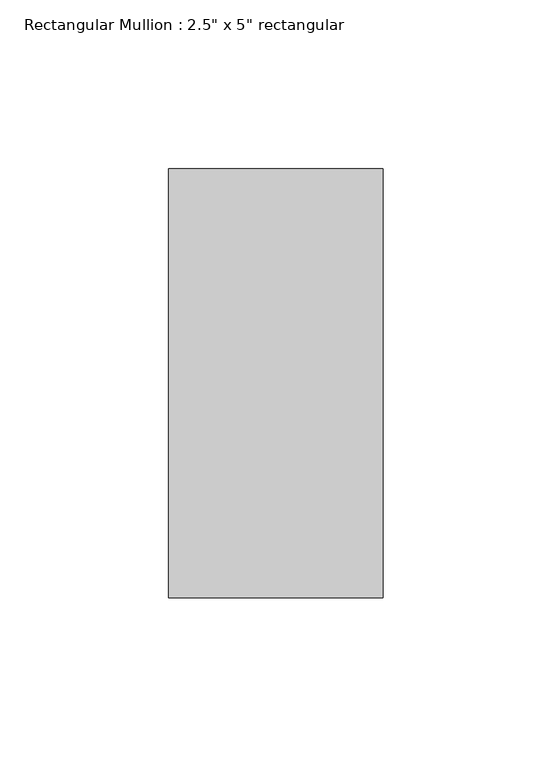
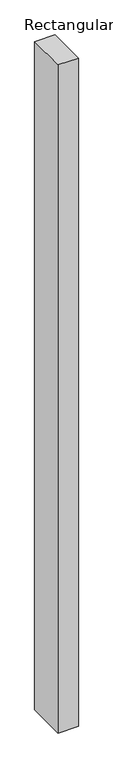
"""IFC4 building model written with IfcOpenShell, lengths in millimetres: member geometry."""

from ifc_helpers import new_model, si_unit, frame, origin, place, context, project, spatial, polyline, outline, extrude, source, transform, mapped, element, save


def member_acd63386(model_context):
    return source(origin(), model_context, "Body", "SweptSolid", [
        extrude(outline(polyline([(31.75, 63.5), (31.75, -63.5), (-31.75, -63.5), (-31.75, 63.5), (31.75, 63.5)])), frame((0.0, 0.0, -2214.7649104), z_axis=(0.0, 0.0, 1.0), x_axis=(1.0, 0.0, 0.0)), (0.0, 0.0, 1.0), 2214.7649104),
    ])


if __name__ == "__main__":
    model = new_model("IFC4")
    model_context = context("Model", 3, world=origin())
    ifc_project = project(units=[si_unit("LENGTHUNIT", "METRE", prefix="MILLI")], contexts=[model_context])
    site = spatial("IfcSite", under=ifc_project)
    building = spatial("IfcBuilding", under=site)
    placement = place(None, origin())
    member_shape = member_acd63386(model_context)
    element("IfcMember", 1, ObjectType="Rectangular Mullion : 2.5\" x 5\" rectangular", at=placement, inside=building, context=model_context, shape_type="MappedRepresentation", body=[
        mapped(member_shape, transform((0.0, 0.0, 0.0), x_axis=(1.0, 0.0, 0.0), y_axis=(0.0, 1.0, 0.0), z_axis=(0.0, 0.0, 1.0))),
    ])
    save(model, "model.ifc")

# Revit data of these elements
# Type "Rectangular Mullion : 2.5\" x 5\" rectangular"
#   built-in parameter 1007304 = 0.416667 (stored number, unit not read)
#   built-in parameter 1007301 = 0.104167 (stored number, unit not read)
#   built-in parameter 1007300 = 0.104167 (stored number, unit not read)
# Element 1 (IfcMember, "Rectangular Mullion : 2.5\" x 5\" rectangular")
#   Materials on its faces: "Aluminum"
# Materials
#   "Aluminum": class "Metal", colour RGB 247 247 247, transparency 0, Description = "Aluminum 6061", Cost = 0
